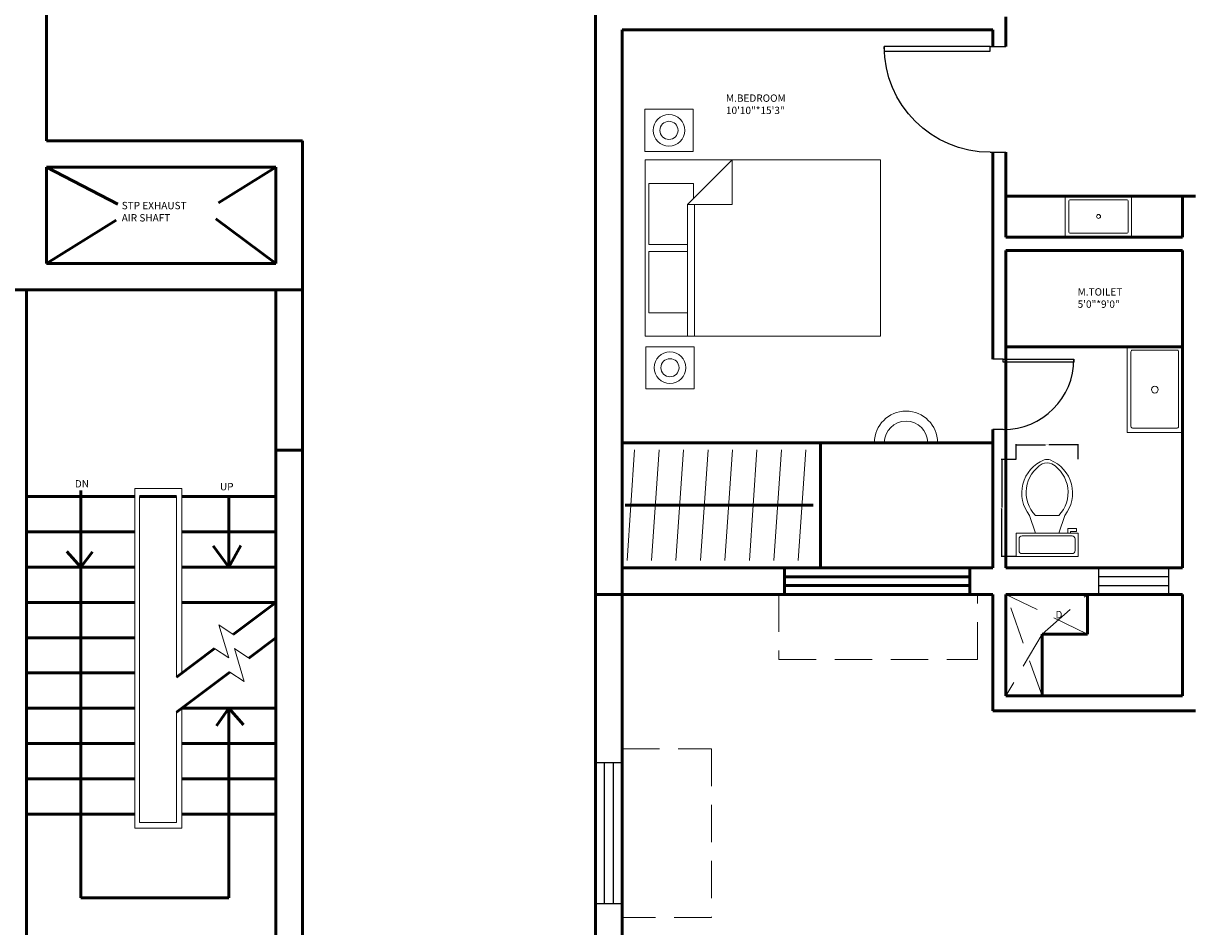
# Model space of a CAD drawing. Units: inches. Extents: x 291 to 2631, y 456 to 2623.
# Tile 17 of 22: x 1974 to 2370, y 1538 to 1845. Entities that reach past the tile are written whole.
import ezdxf

# ---------------------------------------------------------------- set-up
doc = ezdxf.new("R2010")
doc.units = ezdxf.units.IN
doc.linetypes.add('DASHED', pattern=[19.05, 12.7, -6.35])
for name, color, linetype, lineweight in [('A-ANNO-DIMS', 2, 'Continuous', 18), ('A-ANNO-TEXT', 3, 'Continuous', 25), ('A-AREA-IDEN', 7, 'Continuous', 25), ('A-DOOR', 3, 'Continuous', 25), ('A-FLOR-FIXT', 9, 'Continuous', 18), ('A-FLOR-OVHD', 1, 'DASHED', 18), ('A-FURN', 8, 'Continuous', 18), ('A-GLAZ', 4, 'Continuous', 25), ('A-WALL', 7, 'Continuous', 50)]:
    doc.layers.add(name, color=color, linetype=linetype, lineweight=lineweight)
doc.styles.get("Standard").update_dxf_attribs({"font": 'arial.ttf'})
doc.dimstyles.get("Standard").update_dxf_attribs({"dimtxt": 0.18, "dimasz": 0.18, "dimexe": 0.18, "dimexo": 0.0625, "dimgap": 0.09, "dimtad": 0, "dimtih": 1, "dimtoh": 1, "dimdec": 4, "dimzin": 0, "dimdsep": 46, "dimtxsty": 'Standard', "dimcen": 0.09, "dimadec": 0, "dimazin": 0, "dimtfac": 1, "dimtdec": 4, "dimtofl": 0, "dimtmove": 0, "dimatfit": 3, "dimfxl": 1, "dimtolj": 1, "dimtzin": 0, "dimarcsym": 0})

# ---------------------------------------------------------------- blocks, each defined once
blk = doc.blocks.new('Bed - Queen')
for p, q in [((0, -80.00003), (0, 0)), ((0, 0), (59.99999, 0)), ((59.99999, 0), (59.99999, -80.00003)), ((7.99999, -1.2), (28.79998, -1.2)), ((7.99999, -14.4), (7.99999, -1.2)), ((28.79998, -1.2), (28.79998, -14.4)), ((31.19999, -1.2), (51.99999, -1.2)), ((31.19999, -14.4), (31.19999, -1.2)), ((51.99999, -1.2), (51.99999, -16.4)), ((0, -14.4), (44.8, -14.4)), ((59.99999, -29.6), (44.8, -14.4)), ((44.8, -14.4), (44.8, -29.6)), ((44.8, -16.8), (0, -16.8)), ((51.99999, -16.4), (46.79936, -16.4)), ((44.8, -29.6), (59.99999, -29.6)), ((59.99999, -80.00003), (0, -80.00003))]:
    blk.add_line(p, q)
blk = doc.blocks.new('Toilet - top')
for p, q in [((9.5, -6), (9.5, -2)), ((-10, -8.5), (-8, -8.5)), ((-10, -9.5), (-10, -8.5)), ((-7, -9.5), (-10, -9.5)), ((-8, -8.5), (-8, -8)), ((-7, -8), (-7, -9.5)), ((-4, -8), (-6, -14)), ((4, -8), (6, -14)), ((4, -14), (-4, -14))]:
    blk.add_line(p, q)
blk.add_lwpolyline([(10.5, -8), (10.5, 0), (-10.5, 0), (-10.5, -8)], close=True)
for points in [[(-9.5, -2), (-9.5, -6)], [(8.5, -1), (-8.5, -1)], [(-8.5, -7), (8.5, -7)]]:
    blk.add_lwpolyline(points)
for centre, radius, start, end in [((-8.62, -1.88), 0.884, 81.8699, 188.1301), ((8.62, -1.88), 0.884, 351.8699, 98.1301), ((-8.62, -6.12), 0.884, 171.8699, 278.1301), ((8.62, -6.12), 0.884, 261.8699, 8.1301), ((3.52, -21.58), 12.17, 141.4691, 247.9714), ((4.2, -21.82), 11.33, 136.3677, 238.9468), ((-3.52, -21.58), 12.17, 292.0284, 38.5307), ((-4.2, -21.82), 11.33, 301.053, 43.6321), ((0, -27.88), 4, 245.7318, 294.2682), ((0, -29), 4, 254.8605, 285.1395)]:
    blk.add_arc(centre, radius, start, end)
blk = doc.blocks.new('*U2')
for p, q in [((0, 0), (0, -6)), ((40, 0), (40, -6))]:
    blk.add_line(p, q)
blk.add_lwpolyline([(0, 0), (0, 40), (1.75, 40), (1.75, 0)], close=True)
blk.add_arc((0, 0), 40, 0, 90)
blk = doc.blocks.new('WIN-1200')
for p, q in [((0, 0), (0, 48)), ((0, 48), (9, 48)), ((3, 0), (3, 48)), ((6, 48), (6, 0)), ((9, 48), (9, 0)), ((9, 0), (0, 0))]:
    blk.add_line(p, q)
blk = doc.blocks.new('WIN-600')
for p, q in [((24, 9), (0, 9)), ((0, 9), (0, 0)), ((24, 0), (24, 9)), ((24, 6), (0, 6)), ((0, 3), (24, 3)), ((0, 0), (24, 0))]:
    blk.add_line(p, q)
blk = doc.blocks.new('*D30')
at = {"layer": 'A-ANNO-DIMS', "color": 0, "lineweight": -2, "transparency": 16777216}
for p, q in [((2311.15, 1696.58), (2306.08, 1696.58)), ((2306.26, 1696.4), (2306.26, 1680.24)), ((2306.26, 1663.71), (2306.26, 1679.87)), ((2311.15, 1663.53), (2306.08, 1663.53))]:
    blk.add_line(p, q, dxfattribs=at)
at = {"layer": 'A-ANNO-DIMS', "color": 0, "transparency": 16777216}
for points in [[(2306.23, 1696.4), (2306.29, 1696.4), (2306.26, 1696.58)], [(2306.23, 1663.71), (2306.29, 1663.71), (2306.26, 1663.53)]]:
    blk.add_solid(points, dxfattribs=at)
at = {"layer": 'DEFPOINTS', "color": 0, "transparency": 16777216}
for p in [(2311.21, 1696.58), (2306.26, 1663.53), (2311.21, 1663.53)]:
    blk.add_point(p, dxfattribs=at)
at = {"layer": 'A-ANNO-DIMS', "color": 0, "transparency": 16777216, "insert": (2306.26, 1680.06), "char_height": 0.18, "attachment_point": 5}
blk.add_mtext('\\A1;WC 33 TYP.', dxfattribs=at)
blk = doc.blocks.new('*D31')
at = {"layer": 'A-ANNO-DIMS', "color": 0, "lineweight": -2, "transparency": 16777216}
for p, q in [((2311.21, 1696.64), (2311.21, 1701.72)), ((2311.39, 1701.54), (2321.18, 1701.54)), ((2332.03, 1701.54), (2322.24, 1701.54)), ((2332.21, 1696.64), (2332.21, 1701.72))]:
    blk.add_line(p, q, dxfattribs=at)
at = {"layer": 'A-ANNO-DIMS', "color": 0, "transparency": 16777216}
for points in [[(2311.39, 1701.57), (2311.39, 1701.51), (2311.21, 1701.54)], [(2332.03, 1701.57), (2332.03, 1701.51), (2332.21, 1701.54)]]:
    blk.add_solid(points, dxfattribs=at)
at = {"layer": 'DEFPOINTS', "color": 0, "transparency": 16777216}
for p in [(2311.21, 1701.54), (2311.21, 1696.58), (2332.21, 1696.58)]:
    blk.add_point(p, dxfattribs=at)
at = {"layer": 'A-ANNO-DIMS', "color": 0, "transparency": 16777216, "insert": (2321.71, 1701.54), "char_height": 0.18, "attachment_point": 5}
blk.add_mtext('\\A1;21 TYP.', dxfattribs=at)

msp = doc.modelspace()

# ---------------------------------------------------------------- linework, layer by layer
at = {"layer": 'A-FLOR-OVHD'}
for p, q in [((2230.48, 1650.64), (2230.48, 1628.48)), ((2298.03, 1628.48), (2298.03, 1650.64)), ((2319.97, 1616.15), (2307.71, 1650.64)), ((2335.42, 1637.17), (2307.71, 1650.64)), ((2319.97, 1637.17), (2335.42, 1650.64)), ((2319.97, 1637.17), (2307.71, 1616.15)), ((2230.48, 1628.48), (2298.03, 1628.48)), ((2177.21, 1598.14), (2207.65, 1598.14)), ((2207.65, 1598.14), (2207.65, 1540.74)), ((2207.65, 1540.74), (2177.21, 1540.74))]:
    msp.add_line(p, q, dxfattribs=at)
at = {"layer": 'A-FURN'}
for p, q in [((2178.9, 1662.18), (2181.47, 1699.82)), ((2187.21, 1662.18), (2189.78, 1699.82)), ((2195.52, 1662.18), (2198.09, 1699.82)), ((2203.83, 1662.18), (2206.41, 1699.82)), ((2212.15, 1662.18), (2214.72, 1699.82)), ((2220.46, 1662.18), (2223.03, 1699.82)), ((2228.77, 1662.18), (2231.34, 1699.82)), ((2237.08, 1662.18), (2239.66, 1699.82))]:
    msp.add_line(p, q, dxfattribs=at)
for points in [[(2184.89, 1815.63), (2201.38, 1815.63), (2201.38, 1801.33), (2184.89, 1801.33)], [(2327.88, 1786.14), (2350.44, 1786.14), (2350.44, 1772.14), (2327.88, 1772.14)], [(2185.22, 1734.9), (2201.71, 1734.9), (2201.71, 1720.6), (2185.22, 1720.6)], [(2367.71, 1734.86), (2348.96, 1734.86), (2348.96, 1705.73), (2367.71, 1705.73)]]:
    msp.add_lwpolyline(points, close=True, dxfattribs=at)
for points in [[(2329.59, 1784.85), (2348.79, 1784.85, -0.414214), (2349.29, 1784.35), (2349.29, 1774.03, -0.414214), (2348.79, 1773.53), (2329.59, 1773.53, -0.414214), (2329.09, 1774.03), (2329.09, 1784.35, -0.414214)], [(2350.72, 1733.71), (2365.92, 1733.71, -0.414214), (2366.42, 1733.21), (2366.42, 1707.74, -0.414214), (2365.92, 1707.24), (2350.72, 1707.24, -0.414214), (2350.22, 1707.74), (2350.22, 1733.21, -0.414214)]]:
    msp.add_lwpolyline(points, format="xyb", close=True, dxfattribs=at)
for points in [[(2027.5, 1611.94), (2027.5, 1571.21), (2011.51, 1571.21), (2011.51, 1686.66), (2027.5, 1686.66), (2027.5, 1623.94)], [(2025.65, 1610.55), (2025.65, 1573.03), (2013.1, 1573.03), (2013.1, 1683.94)], [(2025.65, 1683.94), (2025.65, 1622.55)], [(2037.22, 1631.23), (2038.6, 1632.27), (2043.49, 1629.07), (2040.1, 1640.26), (2044.99, 1637.07), (2046.37, 1638.1)], [(2041.57, 1622.5), (2043.85, 1624.21), (2048.75, 1621.01), (2045.36, 1632.21), (2050.25, 1629.01), (2052.54, 1630.72)]]:
    msp.add_lwpolyline(points, dxfattribs=at)
for centre, radius in [((2193.14, 1808.48), 5.39), ((2193.14, 1808.48), 3.08), ((2339.19, 1779.19), 0.682), ((2193.47, 1727.75), 5.39), ((2193.47, 1727.75), 3.08), ((2358.34, 1720.3), 1.15)]:
    msp.add_circle(centre, radius, dxfattribs=at)
for radius in [10.73, 7.37]:
    msp.add_arc((2273.73, 1702.26), radius, 0, 180, dxfattribs=at)
at = {"layer": 'A-WALL'}
for p, q in [((1981.49, 2156.24), (1981.49, 1804.93)), ((2168.21, 1876.71), (2168.21, 1650.64)), ((2307.71, 1847.14), (2307.71, 1837.02)), ((2177.21, 1842.64), (2303.21, 1842.64)), ((2177.21, 1842.64), (2177.21, 1659.64)), ((2303.21, 1842.64), (2303.21, 1837.02)), ((2068.49, 1804.93), (1981.49, 1804.93)), ((2068.49, 1754.24), (2068.49, 1804.93)), ((2303.21, 1801.02), (2303.21, 1730.71)), ((2307.71, 1801.02), (2307.71, 1772.14)), ((2059.49, 1795.93), (1981.49, 1795.93)), ((1981.49, 1795.93), (1981.49, 1763.24)), ((1981.49, 1795.93), (2005.77, 1783.41)), ((2059.49, 1795.93), (2039.98, 1783.83)), ((2059.49, 1763.24), (2059.49, 1795.93)), ((2367.71, 1786.14), (2307.71, 1786.14)), ((2372.21, 1786.14), (2367.71, 1786.14)), ((2367.71, 1786.14), (2367.71, 1772.14)), ((1981.49, 1763.24), (2005.16, 1777.91)), ((2059.49, 1763.24), (2039.09, 1778.39)), ((2307.71, 1772.14), (2367.71, 1772.14)), ((2307.71, 1767.64), (2367.71, 1767.64)), ((2307.71, 1767.64), (2307.71, 1659.64)), ((2367.71, 1767.64), (2367.71, 1659.64)), ((1981.49, 1763.24), (2059.49, 1763.24)), ((1981.49, 1754.24), (1808.01, 1754.24)), ((1974.72, 1754.24), (1974.72, 1467.32)), ((1981.49, 1754.24), (2068.49, 1754.24)), ((2059.49, 1754.24), (2059.49, 1490.6)), ((2068.49, 1754.24), (2068.49, 1489.98)), ((2307.71, 1734.86), (2367.71, 1734.86)), ((2303.21, 1706.71), (2303.21, 1659.64)), ((2177.21, 1702.26), (2303.21, 1702.26)), ((2244.68, 1702.26), (2244.68, 1659.64)), ((2059.49, 1699.72), (2068.49, 1699.72)), ((1993.11, 1685.96), (1993.11, 1547.47)), ((1974.72, 1683.94), (2011.51, 1683.94)), ((2013.1, 1683.94), (2025.65, 1683.94)), ((2027.5, 1683.94), (2059.49, 1683.94)), ((2043.49, 1683.94), (2043.49, 1659.94)), ((2178.25, 1681), (2242.15, 1681)), ((1974.72, 1671.94), (2011.51, 1671.94)), ((2027.5, 1671.94), (2059.49, 1671.94)), ((1993.11, 1659.94), (1988.42, 1665.26)), ((1993.11, 1659.94), (1997.18, 1665.19)), ((2043.49, 1659.94), (2038.2, 1667.13)), ((2043.49, 1659.94), (2047.62, 1667.29)), ((1974.72, 1659.94), (2011.51, 1659.94)), ((2027.5, 1659.94), (2059.49, 1659.94)), ((2177.21, 1659.64), (2303.21, 1659.64)), ((2177.21, 1659.64), (2177.21, 1498.02)), ((2232.44, 1659.64), (2303.21, 1659.64)), ((2232.44, 1650.64), (2232.44, 1659.64)), ((2232.44, 1656.64), (2295.4, 1656.64)), ((2295.4, 1659.64), (2295.4, 1650.64)), ((2307.71, 1659.64), (2367.71, 1659.64)), ((2295.4, 1653.64), (2232.44, 1653.64)), ((2168.21, 1650.64), (2303.21, 1650.64)), ((2168.21, 1650.64), (2168.21, 1112.52)), ((2303.21, 1650.64), (2232.44, 1650.64)), ((2303.21, 1650.64), (2303.21, 1611.04)), ((2307.71, 1650.64), (2307.71, 1616.15)), ((2307.71, 1650.64), (2367.71, 1650.64)), ((2335.42, 1637.17), (2335.42, 1650.64)), ((2367.71, 1616.15), (2367.71, 1650.64)), ((1974.72, 1647.94), (2011.51, 1647.94)), ((2027.5, 1647.94), (2059.49, 1647.94)), ((2044.99, 1637.07), (2059.49, 1647.94)), ((2319.97, 1616.15), (2319.97, 1637.17)), ((2319.97, 1637.17), (2335.42, 1637.17)), ((1974.72, 1635.94), (2011.51, 1635.94)), ((2050.25, 1629.01), (2059.49, 1635.94)), ((2025.65, 1622.55), (2038.6, 1632.27)), ((1974.72, 1623.94), (2011.51, 1623.94)), ((2025.65, 1610.55), (2043.85, 1624.21)), ((2307.71, 1616.15), (2367.71, 1616.15)), ((1974.72, 1611.94), (2011.51, 1611.94)), ((2027.5, 1611.94), (2059.49, 1611.94)), ((2043.49, 1611.94), (2039.25, 1606)), ((2043.49, 1547.47), (2043.49, 1611.94)), ((2043.49, 1611.94), (2048.44, 1606.34)), ((2303.21, 1611.04), (2372.21, 1611.04)), ((1974.72, 1599.94), (2011.51, 1599.94)), ((2027.5, 1599.94), (2059.49, 1599.94)), ((1974.72, 1587.94), (2011.51, 1587.94)), ((2027.5, 1587.94), (2059.49, 1587.94)), ((1974.72, 1575.94), (2011.51, 1575.94)), ((2027.5, 1575.94), (2059.49, 1575.94)), ((1993.11, 1547.47), (2043.49, 1547.47))]:
    msp.add_line(p, q, dxfattribs=at)

# ---------------------------------------------------------------- block references
at = {"layer": 'A-DOOR'}
for p, xscale, yscale, zscale, rotation in [((2302.31, 1837.02), -0.9, 0.9, 0.9, 90), ((2306.81, 1730.71), 0.6, 0.6, 0.6, 270)]:
    msp.add_blockref('*U2', p, dxfattribs=dict(at, xscale=xscale, yscale=yscale, zscale=zscale, rotation=rotation))
at = {"layer": 'A-FLOR-FIXT', "rotation": 180}
msp.add_blockref('Toilet - top', (2321.71, 1663.53), dxfattribs=at)
at = {"layer": 'A-FURN', "rotation": 90}
msp.add_blockref('Bed - Queen', (2185.04, 1738.45), dxfattribs=at)
at = {"layer": 'A-GLAZ', "rotation": 180}
for name, p in [('WIN-600', (2363.14, 1659.64)), ('WIN-1200', (2177.21, 1593.46))]:
    msp.add_blockref(name, p, dxfattribs=at)

# ---------------------------------------------------------------- texts
at = {"layer": 'A-ANNO-TEXT', "char_height": 2.5, "attachment_point": 1}
for s, width, insert in [('DN', 7.4274, (1991.13, 1689.53)), ('UP', 6.7235, (2040.46, 1688.55)), ('D', 2.6921, (2324.56, 1645.04))]:
    msp.add_mtext_dynamic_manual_height_columns(s, width=width, gutter_width=12.5, heights=[0], dxfattribs=dict(at, insert=insert))
at = {"layer": 'A-AREA-IDEN', "char_height": 2.5, "attachment_point": 1}
for s, width, insert in [('M.BEDROOM\\P10\'10"*15\'3"', 45.6618, (2212.51, 1820.69)), ('STP EXHAUST\\PAIR SHAFT', 29.5412, (2007.06, 1784.15)), ('M.TOILET\\P5\'0"*9\'0"', 47.5304, (2332.09, 1754.79))]:
    msp.add_mtext_dynamic_manual_height_columns(s, width=width, gutter_width=12.5, heights=[0], dxfattribs=dict(at, insert=insert))

# ---------------------------------------------------------------- dimensions: what is measured, and where the dimension line sits
at = {"layer": 'A-ANNO-DIMS'}
for base, p1, p2, angle, text, picture, middle in [((2311.21, 1701.54), (2332.21, 1696.58), (2311.21, 1696.58), 180, '<> TYP.', '*D31', (2321.71, 1701.54)), ((2306.26, 1663.53), (2311.21, 1696.58), (2311.21, 1663.53), 270, 'WC <> TYP.', '*D30', (2306.26, 1680.06))]:
    dim = msp.add_linear_dim(base=base, p1=p1, p2=p2, angle=angle, text=text, dimstyle='Standard', override={"dimdec": 0, "dimlfac": 1, "dimrnd": 0, "dimzin": 0, "dimdsep": 46, "dimlunit": 2}, dxfattribs=at)
    dim.commit()
    dim.dimension.update_dxf_attribs({"geometry": picture, "text_midpoint": middle})

doc.saveas('drawing.dxf')
